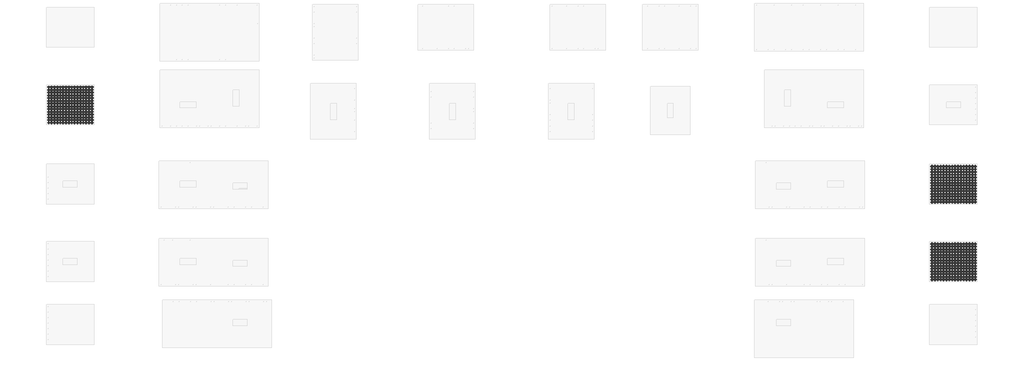
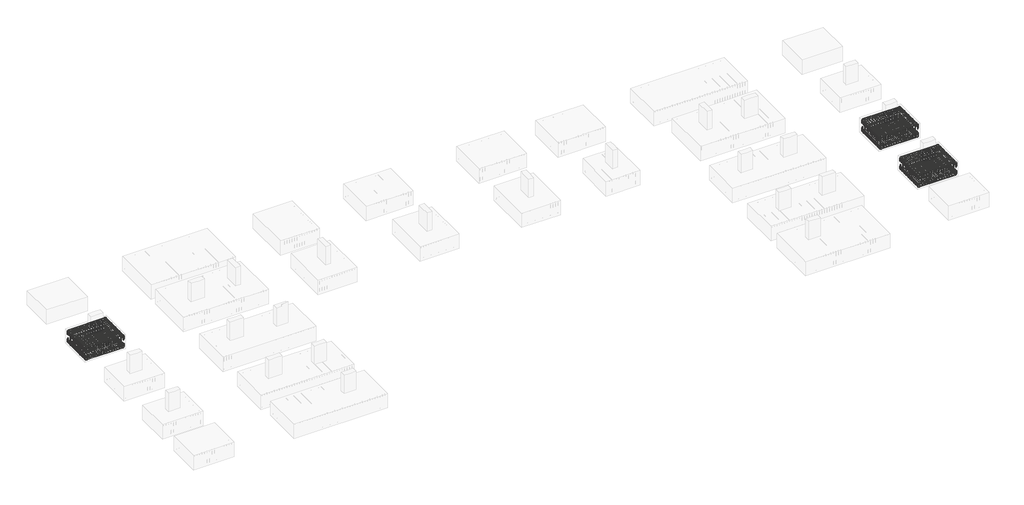
# One storey, part 9 of 21: 12 reinforcing bars.
"""IFC4 building model written with IfcOpenShell, lengths in millimetres."""

from ifc_helpers import new_model, si_unit, point, frame, origin, place, context, project, spatial, polyline, circle_curve, trimmed, segment, composite_curve, source, transform, mapped, element, save
from ifc_brep_helpers import swept_disk

model = new_model("IFC4")

# Units and contexts
model_context = context("Model", 3, world=origin())
ifc_project = project(units=[si_unit("LENGTHUNIT", "METRE", prefix="MILLI")], contexts=[model_context])

# Site, building, storey
site = spatial("IfcSite", under=ifc_project)
building = spatial("IfcBuilding", under=site)
storey = spatial("IfcBuildingStorey", under=building, Elevation=-1100.0)

# Reinforcing bars
placement = place(None, origin())
reinforcing_bar_shape = source(origin(), model_context, "Body", "SolidModel", [
    swept_disk(composite_curve([segment(polyline([(-23061.1351198, 4447.9216575, -1700.0), (-23061.1351198, 4447.9216575, -1882.5)]), True, "CONTINUOUS"), segment(trimmed(circle_curve(frame((-23118.6351198, 4447.9216575, -1882.5), z_axis=(0.0, 1.0, 0.0), x_axis=(57.5, 0.0, 0.0)), 57.5), [point((-23061.1351198, 4447.9216575, -1882.5))], [point((-23118.6351198, 4447.9216575, -1940.0))], True, "CARTESIAN"), True, "CONTINUOUS"), segment(polyline([(-23118.6351198, 4447.9216575, -1940.0), (-25283.6351198, 4447.9216575, -1940.0)]), True, "CONTINUOUS"), segment(trimmed(circle_curve(frame((-25283.6351198, 4447.9216575, -1882.5), z_axis=(0.0, 1.0, 0.0), x_axis=(0.0, 0.0, -57.5)), 57.5), [point((-25283.6351198, 4447.9216575, -1940.0))], [point((-25341.1351198, 4447.9216575, -1882.5))], True, "CARTESIAN"), True, "CONTINUOUS"), segment(polyline([(-25341.1351198, 4447.9216575, -1882.5), (-25341.1351198, 4447.9216575, -1700.0)]), True, "CONTINUOUS")], self_intersect=False), 10.0),
])
element("IfcReinforcingBar", 1, at=placement, inside=storey, context=model_context, shape_type="MappedRepresentation", body=[
    mapped(reinforcing_bar_shape, transform((0.0, 0.0, 0.0), x_axis=(1.0, 0.0, 0.0), y_axis=(0.0, 1.0, 0.0), z_axis=(0.0, 0.0, 1.0))),
    mapped(reinforcing_bar_shape, transform((0.0, -138.5928916, 0.0), x_axis=(1.0, 0.0, 0.0), y_axis=(0.0, 1.0, 0.0), z_axis=(0.0, 0.0, 1.0))),
    mapped(reinforcing_bar_shape, transform((0.0, -277.1857833, 0.0), x_axis=(1.0, 0.0, 0.0), y_axis=(0.0, 1.0, 0.0), z_axis=(0.0, 0.0, 1.0))),
    mapped(reinforcing_bar_shape, transform((0.0, -415.7786749, 0.0), x_axis=(1.0, 0.0, 0.0), y_axis=(0.0, 1.0, 0.0), z_axis=(0.0, 0.0, 1.0))),
    mapped(reinforcing_bar_shape, transform((0.0, -554.3715666, 0.0), x_axis=(1.0, 0.0, 0.0), y_axis=(0.0, 1.0, 0.0), z_axis=(0.0, 0.0, 1.0))),
    mapped(reinforcing_bar_shape, transform((0.0, -692.9644582, 0.0), x_axis=(1.0, 0.0, 0.0), y_axis=(0.0, 1.0, 0.0), z_axis=(0.0, 0.0, 1.0))),
    mapped(reinforcing_bar_shape, transform((0.0, -831.5573499, 0.0), x_axis=(1.0, 0.0, 0.0), y_axis=(0.0, 1.0, 0.0), z_axis=(0.0, 0.0, 1.0))),
    mapped(reinforcing_bar_shape, transform((0.0, -970.1502415, 0.0), x_axis=(1.0, 0.0, 0.0), y_axis=(0.0, 1.0, 0.0), z_axis=(0.0, 0.0, 1.0))),
    mapped(reinforcing_bar_shape, transform((0.0, -1108.7431331, 0.0), x_axis=(1.0, 0.0, 0.0), y_axis=(0.0, 1.0, 0.0), z_axis=(0.0, 0.0, 1.0))),
    mapped(reinforcing_bar_shape, transform((0.0, -1247.3360248, 0.0), x_axis=(1.0, 0.0, 0.0), y_axis=(0.0, 1.0, 0.0), z_axis=(0.0, 0.0, 1.0))),
    mapped(reinforcing_bar_shape, transform((0.0, -1385.9289164, 0.0), x_axis=(1.0, 0.0, 0.0), y_axis=(0.0, 1.0, 0.0), z_axis=(0.0, 0.0, 1.0))),
    mapped(reinforcing_bar_shape, transform((0.0, -1524.5218081, 0.0), x_axis=(1.0, 0.0, 0.0), y_axis=(0.0, 1.0, 0.0), z_axis=(0.0, 0.0, 1.0))),
    mapped(reinforcing_bar_shape, transform((0.0, -1663.1146997, 0.0), x_axis=(1.0, 0.0, 0.0), y_axis=(0.0, 1.0, 0.0), z_axis=(0.0, 0.0, 1.0))),
    mapped(reinforcing_bar_shape, transform((0.0, -1801.7075913, 0.0), x_axis=(1.0, 0.0, 0.0), y_axis=(0.0, 1.0, 0.0), z_axis=(0.0, 0.0, 1.0))),
])
reinforcing_bar_2_shape = source(origin(), model_context, "Body", "SolidModel", [
    swept_disk(composite_curve([segment(polyline([(-25343.1851198, 4447.9216575, -1400.0), (-25343.1851198, 4447.9216575, -1213.4)]), True, "CONTINUOUS"), segment(trimmed(circle_curve(frame((-25287.7351198, 4447.9216575, -1213.4), z_axis=(0.0, 1.0, 0.0), x_axis=(-55.45000000000073, 0.0, 0.0)), 55.45), [point((-25343.1851198, 4447.9216575, -1213.4))], [point((-25287.7351198, 4447.9216575, -1157.95))], True, "CARTESIAN"), True, "CONTINUOUS"), segment(polyline([(-25287.7351198, 4447.9216575, -1157.95), (-23114.5351198, 4447.9216575, -1157.95)]), True, "CONTINUOUS"), segment(trimmed(circle_curve(frame((-23114.5351198, 4447.9216575, -1213.4), z_axis=(0.0, 1.0, 0.0), x_axis=(0.0, 0.0, 55.450000000000045)), 55.45), [point((-23114.5351198, 4447.9216575, -1157.95))], [point((-23059.0851198, 4447.9216575, -1213.4))], True, "CARTESIAN"), True, "CONTINUOUS"), segment(polyline([(-23059.0851198, 4447.9216575, -1213.4), (-23059.0851198, 4447.9216575, -1400.0)]), True, "CONTINUOUS")], self_intersect=False), 7.95),
])
element("IfcReinforcingBar", 2, at=placement, inside=storey, context=model_context, shape_type="MappedRepresentation", body=[
    mapped(reinforcing_bar_2_shape, transform((0.0, 0.0, 0.0), x_axis=(1.0, 0.0, 0.0), y_axis=(0.0, 1.0, 0.0), z_axis=(0.0, 0.0, 1.0))),
    mapped(reinforcing_bar_2_shape, transform((0.0, -138.5928916, 0.0), x_axis=(1.0, 0.0, 0.0), y_axis=(0.0, 1.0, 0.0), z_axis=(0.0, 0.0, 1.0))),
    mapped(reinforcing_bar_2_shape, transform((0.0, -277.1857833, 0.0), x_axis=(1.0, 0.0, 0.0), y_axis=(0.0, 1.0, 0.0), z_axis=(0.0, 0.0, 1.0))),
    mapped(reinforcing_bar_2_shape, transform((0.0, -415.7786749, 0.0), x_axis=(1.0, 0.0, 0.0), y_axis=(0.0, 1.0, 0.0), z_axis=(0.0, 0.0, 1.0))),
    mapped(reinforcing_bar_2_shape, transform((0.0, -554.3715666, 0.0), x_axis=(1.0, 0.0, 0.0), y_axis=(0.0, 1.0, 0.0), z_axis=(0.0, 0.0, 1.0))),
    mapped(reinforcing_bar_2_shape, transform((0.0, -692.9644582, 0.0), x_axis=(1.0, 0.0, 0.0), y_axis=(0.0, 1.0, 0.0), z_axis=(0.0, 0.0, 1.0))),
    mapped(reinforcing_bar_2_shape, transform((0.0, -831.5573499, 0.0), x_axis=(1.0, 0.0, 0.0), y_axis=(0.0, 1.0, 0.0), z_axis=(0.0, 0.0, 1.0))),
    mapped(reinforcing_bar_2_shape, transform((0.0, -970.1502415, 0.0), x_axis=(1.0, 0.0, 0.0), y_axis=(0.0, 1.0, 0.0), z_axis=(0.0, 0.0, 1.0))),
    mapped(reinforcing_bar_2_shape, transform((0.0, -1108.7431331, 0.0), x_axis=(1.0, 0.0, 0.0), y_axis=(0.0, 1.0, 0.0), z_axis=(0.0, 0.0, 1.0))),
    mapped(reinforcing_bar_2_shape, transform((0.0, -1247.3360248, 0.0), x_axis=(1.0, 0.0, 0.0), y_axis=(0.0, 1.0, 0.0), z_axis=(0.0, 0.0, 1.0))),
    mapped(reinforcing_bar_2_shape, transform((0.0, -1385.9289164, 0.0), x_axis=(1.0, 0.0, 0.0), y_axis=(0.0, 1.0, 0.0), z_axis=(0.0, 0.0, 1.0))),
    mapped(reinforcing_bar_2_shape, transform((0.0, -1524.5218081, 0.0), x_axis=(1.0, 0.0, 0.0), y_axis=(0.0, 1.0, 0.0), z_axis=(0.0, 0.0, 1.0))),
    mapped(reinforcing_bar_2_shape, transform((0.0, -1663.1146997, 0.0), x_axis=(1.0, 0.0, 0.0), y_axis=(0.0, 1.0, 0.0), z_axis=(0.0, 0.0, 1.0))),
    mapped(reinforcing_bar_2_shape, transform((0.0, -1801.7075913, 0.0), x_axis=(1.0, 0.0, 0.0), y_axis=(0.0, 1.0, 0.0), z_axis=(0.0, 0.0, 1.0))),
])
reinforcing_bar_3_shape = source(origin(), model_context, "Body", "SolidModel", [
    swept_disk(composite_curve([segment(polyline([(-23110.9192838, 4486.2204288, -1428.1111113), (-23110.9192838, 4486.2204288, -1241.5111113)]), True, "CONTINUOUS"), segment(trimmed(circle_curve(frame((-23110.9192838, 4430.7704288, -1241.5111113), z_axis=(1.0, 0.0, 0.0), x_axis=(0.0, 55.44999999999982, 0.0)), 55.45), [point((-23110.9192838, 4486.2204288, -1241.5111113))], [point((-23110.9192838, 4430.7704288, -1186.0611113))], True, "CARTESIAN"), True, "CONTINUOUS"), segment(polyline([(-23110.9192838, 4430.7704288, -1186.0611113), (-23110.9192838, 2657.5704288, -1186.0611113)]), True, "CONTINUOUS"), segment(trimmed(circle_curve(frame((-23110.9192838, 2657.5704288, -1241.5111113), z_axis=(1.0, 0.0, 0.0), x_axis=(0.0, 0.0, 55.450000000000045)), 55.45), [point((-23110.9192838, 2657.5704288, -1186.0611113))], [point((-23110.9192838, 2602.1204288, -1241.5111113))], True, "CARTESIAN"), True, "CONTINUOUS"), segment(polyline([(-23110.9192838, 2602.1204288, -1241.5111113), (-23110.9192838, 2602.1204288, -1428.1111113)]), True, "CONTINUOUS")], self_intersect=False), 7.95),
])
element("IfcReinforcingBar", 3, at=placement, inside=storey, context=model_context, shape_type="MappedRepresentation", body=[
    mapped(reinforcing_bar_3_shape, transform((0.0, 0.0, 0.0), x_axis=(1.0, 0.0, 0.0), y_axis=(0.0, 1.0, 0.0), z_axis=(0.0, 0.0, 1.0))),
    mapped(reinforcing_bar_3_shape, transform((-145.2528929, 0.0, 0.0), x_axis=(1.0, 0.0, 0.0), y_axis=(0.0, 1.0, 0.0), z_axis=(0.0, 0.0, 1.0))),
    mapped(reinforcing_bar_3_shape, transform((-290.5057858, 0.0, 0.0), x_axis=(1.0, 0.0, 0.0), y_axis=(0.0, 1.0, 0.0), z_axis=(0.0, 0.0, 1.0))),
    mapped(reinforcing_bar_3_shape, transform((-435.7586787, 0.0, 0.0), x_axis=(1.0, 0.0, 0.0), y_axis=(0.0, 1.0, 0.0), z_axis=(0.0, 0.0, 1.0))),
    mapped(reinforcing_bar_3_shape, transform((-581.0115716, 0.0, 0.0), x_axis=(1.0, 0.0, 0.0), y_axis=(0.0, 1.0, 0.0), z_axis=(0.0, 0.0, 1.0))),
    mapped(reinforcing_bar_3_shape, transform((-726.2644645, 0.0, 0.0), x_axis=(1.0, 0.0, 0.0), y_axis=(0.0, 1.0, 0.0), z_axis=(0.0, 0.0, 1.0))),
    mapped(reinforcing_bar_3_shape, transform((-871.5173574, 0.0, 0.0), x_axis=(1.0, 0.0, 0.0), y_axis=(0.0, 1.0, 0.0), z_axis=(0.0, 0.0, 1.0))),
    mapped(reinforcing_bar_3_shape, transform((-1016.7702503, 0.0, 0.0), x_axis=(1.0, 0.0, 0.0), y_axis=(0.0, 1.0, 0.0), z_axis=(0.0, 0.0, 1.0))),
    mapped(reinforcing_bar_3_shape, transform((-1162.0231432, 0.0, 0.0), x_axis=(1.0, 0.0, 0.0), y_axis=(0.0, 1.0, 0.0), z_axis=(0.0, 0.0, 1.0))),
    mapped(reinforcing_bar_3_shape, transform((-1307.276036, 0.0, 0.0), x_axis=(1.0, 0.0, 0.0), y_axis=(0.0, 1.0, 0.0), z_axis=(0.0, 0.0, 1.0))),
    mapped(reinforcing_bar_3_shape, transform((-1452.5289289, 0.0, 0.0), x_axis=(1.0, 0.0, 0.0), y_axis=(0.0, 1.0, 0.0), z_axis=(0.0, 0.0, 1.0))),
    mapped(reinforcing_bar_3_shape, transform((-1597.7818218, 0.0, 0.0), x_axis=(1.0, 0.0, 0.0), y_axis=(0.0, 1.0, 0.0), z_axis=(0.0, 0.0, 1.0))),
    mapped(reinforcing_bar_3_shape, transform((-1743.0347147, 0.0, 0.0), x_axis=(1.0, 0.0, 0.0), y_axis=(0.0, 1.0, 0.0), z_axis=(0.0, 0.0, 1.0))),
    mapped(reinforcing_bar_3_shape, transform((-1888.2876076, 0.0, 0.0), x_axis=(1.0, 0.0, 0.0), y_axis=(0.0, 1.0, 0.0), z_axis=(0.0, 0.0, 1.0))),
    mapped(reinforcing_bar_3_shape, transform((-2033.5405005, 0.0, 0.0), x_axis=(1.0, 0.0, 0.0), y_axis=(0.0, 1.0, 0.0), z_axis=(0.0, 0.0, 1.0))),
    mapped(reinforcing_bar_3_shape, transform((-2178.7933934, 0.0, 0.0), x_axis=(1.0, 0.0, 0.0), y_axis=(0.0, 1.0, 0.0), z_axis=(0.0, 0.0, 1.0))),
])
reinforcing_bar_4_shape = source(origin(), model_context, "Body", "SolidModel", [
    swept_disk(composite_curve([segment(polyline([(-25289.7126773, 4484.1704288, -1669.8442859), (-25289.7126773, 4484.1704288, -1852.3442859)]), True, "CONTINUOUS"), segment(trimmed(circle_curve(frame((-25289.7126773, 4426.6704288, -1852.3442859), z_axis=(-1.0, 0.0, 0.0), x_axis=(0.0, 57.5, 0.0)), 57.5), [point((-25289.7126773, 4484.1704288, -1852.3442859))], [point((-25289.7126773, 4426.6704288, -1909.8442859))], True, "CARTESIAN"), True, "CONTINUOUS"), segment(polyline([(-25289.7126773, 4426.6704288, -1909.8442859), (-25289.7126773, 2661.6704288, -1909.8442859)]), True, "CONTINUOUS"), segment(trimmed(circle_curve(frame((-25289.7126773, 2661.6704288, -1852.3442859), z_axis=(-1.0, 0.0, 0.0), x_axis=(0.0, 0.0, -57.5)), 57.5), [point((-25289.7126773, 2661.6704288, -1909.8442859))], [point((-25289.7126773, 2604.1704288, -1852.3442859))], True, "CARTESIAN"), True, "CONTINUOUS"), segment(polyline([(-25289.7126773, 2604.1704288, -1852.3442859), (-25289.7126773, 2604.1704288, -1669.8442859)]), True, "CONTINUOUS")], self_intersect=False), 10.0),
])
element("IfcReinforcingBar", 4, at=placement, inside=storey, context=model_context, shape_type="MappedRepresentation", body=[
    mapped(reinforcing_bar_4_shape, transform((0.0, 0.0, 0.0), x_axis=(1.0, 0.0, 0.0), y_axis=(0.0, 1.0, 0.0), z_axis=(0.0, 0.0, 1.0))),
    mapped(reinforcing_bar_4_shape, transform((145.2528929, 0.0, 0.0), x_axis=(1.0, 0.0, 0.0), y_axis=(0.0, 1.0, 0.0), z_axis=(0.0, 0.0, 1.0))),
    mapped(reinforcing_bar_4_shape, transform((290.5057858, 0.0, 0.0), x_axis=(1.0, 0.0, 0.0), y_axis=(0.0, 1.0, 0.0), z_axis=(0.0, 0.0, 1.0))),
    mapped(reinforcing_bar_4_shape, transform((435.7586787, 0.0, 0.0), x_axis=(1.0, 0.0, 0.0), y_axis=(0.0, 1.0, 0.0), z_axis=(0.0, 0.0, 1.0))),
    mapped(reinforcing_bar_4_shape, transform((581.0115716, 0.0, 0.0), x_axis=(1.0, 0.0, 0.0), y_axis=(0.0, 1.0, 0.0), z_axis=(0.0, 0.0, 1.0))),
    mapped(reinforcing_bar_4_shape, transform((726.2644645, 0.0, 0.0), x_axis=(1.0, 0.0, 0.0), y_axis=(0.0, 1.0, 0.0), z_axis=(0.0, 0.0, 1.0))),
    mapped(reinforcing_bar_4_shape, transform((871.5173574, 0.0, 0.0), x_axis=(1.0, 0.0, 0.0), y_axis=(0.0, 1.0, 0.0), z_axis=(0.0, 0.0, 1.0))),
    mapped(reinforcing_bar_4_shape, transform((1016.7702503, 0.0, 0.0), x_axis=(1.0, 0.0, 0.0), y_axis=(0.0, 1.0, 0.0), z_axis=(0.0, 0.0, 1.0))),
    mapped(reinforcing_bar_4_shape, transform((1162.0231432, 0.0, 0.0), x_axis=(1.0, 0.0, 0.0), y_axis=(0.0, 1.0, 0.0), z_axis=(0.0, 0.0, 1.0))),
    mapped(reinforcing_bar_4_shape, transform((1307.276036, 0.0, 0.0), x_axis=(1.0, 0.0, 0.0), y_axis=(0.0, 1.0, 0.0), z_axis=(0.0, 0.0, 1.0))),
    mapped(reinforcing_bar_4_shape, transform((1452.5289289, 0.0, 0.0), x_axis=(1.0, 0.0, 0.0), y_axis=(0.0, 1.0, 0.0), z_axis=(0.0, 0.0, 1.0))),
    mapped(reinforcing_bar_4_shape, transform((1597.7818218, 0.0, 0.0), x_axis=(1.0, 0.0, 0.0), y_axis=(0.0, 1.0, 0.0), z_axis=(0.0, 0.0, 1.0))),
    mapped(reinforcing_bar_4_shape, transform((1743.0347147, 0.0, 0.0), x_axis=(1.0, 0.0, 0.0), y_axis=(0.0, 1.0, 0.0), z_axis=(0.0, 0.0, 1.0))),
    mapped(reinforcing_bar_4_shape, transform((1888.2876076, 0.0, 0.0), x_axis=(1.0, 0.0, 0.0), y_axis=(0.0, 1.0, 0.0), z_axis=(0.0, 0.0, 1.0))),
    mapped(reinforcing_bar_4_shape, transform((2033.5405005, 0.0, 0.0), x_axis=(1.0, 0.0, 0.0), y_axis=(0.0, 1.0, 0.0), z_axis=(0.0, 0.0, 1.0))),
    mapped(reinforcing_bar_4_shape, transform((2178.7933934, 0.0, 0.0), x_axis=(1.0, 0.0, 0.0), y_axis=(0.0, 1.0, 0.0), z_axis=(0.0, 0.0, 1.0))),
])
reinforcing_bar_5_shape = source(origin(), model_context, "Body", "SolidModel", [
    swept_disk(composite_curve([segment(polyline([(19239.1673659, -5269.5807999, -1700.0), (19239.1673659, -5269.5807999, -1882.5)]), True, "CONTINUOUS"), segment(trimmed(circle_curve(frame((19296.6673659, -5269.5807999, -1882.5), z_axis=(0.0, -1.0, 0.0), x_axis=(-57.5, 0.0, 0.0)), 57.5), [point((19239.1673659, -5269.5807999, -1882.5))], [point((19296.6673659, -5269.5807999, -1940.0))], True, "CARTESIAN"), True, "CONTINUOUS"), segment(polyline([(19296.6673659, -5269.5807999, -1940.0), (21461.6673659, -5269.5807999, -1940.0)]), True, "CONTINUOUS"), segment(trimmed(circle_curve(frame((21461.6673659, -5269.5807999, -1882.5), z_axis=(0.0, -1.0, 0.0), x_axis=(0.0, 0.0, -57.5)), 57.5), [point((21461.6673659, -5269.5807999, -1940.0))], [point((21519.1673659, -5269.5807999, -1882.5))], True, "CARTESIAN"), True, "CONTINUOUS"), segment(polyline([(21519.1673659, -5269.5807999, -1882.5), (21519.1673659, -5269.5807999, -1700.0)]), True, "CONTINUOUS")], self_intersect=False), 10.0),
])
element("IfcReinforcingBar", 5, at=placement, inside=storey, context=model_context, shape_type="MappedRepresentation", body=[
    mapped(reinforcing_bar_5_shape, transform((0.0, 0.0, 0.0), x_axis=(1.0, 0.0, 0.0), y_axis=(0.0, 1.0, 0.0), z_axis=(0.0, 0.0, 1.0))),
    mapped(reinforcing_bar_5_shape, transform((0.0, 138.5928916, 0.0), x_axis=(1.0, 0.0, 0.0), y_axis=(0.0, 1.0, 0.0), z_axis=(0.0, 0.0, 1.0))),
    mapped(reinforcing_bar_5_shape, transform((0.0, 277.1857833, 0.0), x_axis=(1.0, 0.0, 0.0), y_axis=(0.0, 1.0, 0.0), z_axis=(0.0, 0.0, 1.0))),
    mapped(reinforcing_bar_5_shape, transform((0.0, 415.7786749, 0.0), x_axis=(1.0, 0.0, 0.0), y_axis=(0.0, 1.0, 0.0), z_axis=(0.0, 0.0, 1.0))),
    mapped(reinforcing_bar_5_shape, transform((0.0, 554.3715666, 0.0), x_axis=(1.0, 0.0, 0.0), y_axis=(0.0, 1.0, 0.0), z_axis=(0.0, 0.0, 1.0))),
    mapped(reinforcing_bar_5_shape, transform((0.0, 692.9644582, 0.0), x_axis=(1.0, 0.0, 0.0), y_axis=(0.0, 1.0, 0.0), z_axis=(0.0, 0.0, 1.0))),
    mapped(reinforcing_bar_5_shape, transform((0.0, 831.5573499, 0.0), x_axis=(1.0, 0.0, 0.0), y_axis=(0.0, 1.0, 0.0), z_axis=(0.0, 0.0, 1.0))),
    mapped(reinforcing_bar_5_shape, transform((0.0, 970.1502415, 0.0), x_axis=(1.0, 0.0, 0.0), y_axis=(0.0, 1.0, 0.0), z_axis=(0.0, 0.0, 1.0))),
    mapped(reinforcing_bar_5_shape, transform((0.0, 1108.7431331, 0.0), x_axis=(1.0, 0.0, 0.0), y_axis=(0.0, 1.0, 0.0), z_axis=(0.0, 0.0, 1.0))),
    mapped(reinforcing_bar_5_shape, transform((0.0, 1247.3360248, 0.0), x_axis=(1.0, 0.0, 0.0), y_axis=(0.0, 1.0, 0.0), z_axis=(0.0, 0.0, 1.0))),
    mapped(reinforcing_bar_5_shape, transform((0.0, 1385.9289164, 0.0), x_axis=(1.0, 0.0, 0.0), y_axis=(0.0, 1.0, 0.0), z_axis=(0.0, 0.0, 1.0))),
    mapped(reinforcing_bar_5_shape, transform((0.0, 1524.5218081, 0.0), x_axis=(1.0, 0.0, 0.0), y_axis=(0.0, 1.0, 0.0), z_axis=(0.0, 0.0, 1.0))),
    mapped(reinforcing_bar_5_shape, transform((0.0, 1663.1146997, 0.0), x_axis=(1.0, 0.0, 0.0), y_axis=(0.0, 1.0, 0.0), z_axis=(0.0, 0.0, 1.0))),
    mapped(reinforcing_bar_5_shape, transform((0.0, 1801.7075913, 0.0), x_axis=(1.0, 0.0, 0.0), y_axis=(0.0, 1.0, 0.0), z_axis=(0.0, 0.0, 1.0))),
])
reinforcing_bar_6_shape = source(origin(), model_context, "Body", "SolidModel", [
    swept_disk(composite_curve([segment(polyline([(21521.2173659, -5269.5807999, -1400.0), (21521.2173659, -5269.5807999, -1213.4)]), True, "CONTINUOUS"), segment(trimmed(circle_curve(frame((21465.7673659, -5269.5807999, -1213.4), z_axis=(0.0, -1.0, 0.0), x_axis=(55.45000000000073, 0.0, 0.0)), 55.45), [point((21521.2173659, -5269.5807999, -1213.4))], [point((21465.7673659, -5269.5807999, -1157.95))], True, "CARTESIAN"), True, "CONTINUOUS"), segment(polyline([(21465.7673659, -5269.5807999, -1157.95), (19292.5673659, -5269.5807999, -1157.95)]), True, "CONTINUOUS"), segment(trimmed(circle_curve(frame((19292.5673659, -5269.5807999, -1213.4), z_axis=(0.0, -1.0, 0.0), x_axis=(0.0, 0.0, 55.450000000000045)), 55.45), [point((19292.5673659, -5269.5807999, -1157.95))], [point((19237.1173659, -5269.5807999, -1213.4))], True, "CARTESIAN"), True, "CONTINUOUS"), segment(polyline([(19237.1173659, -5269.5807999, -1213.4), (19237.1173659, -5269.5807999, -1400.0)]), True, "CONTINUOUS")], self_intersect=False), 7.95),
])
element("IfcReinforcingBar", 6, at=placement, inside=storey, context=model_context, shape_type="MappedRepresentation", body=[
    mapped(reinforcing_bar_6_shape, transform((0.0, 0.0, 0.0), x_axis=(1.0, 0.0, 0.0), y_axis=(0.0, 1.0, 0.0), z_axis=(0.0, 0.0, 1.0))),
    mapped(reinforcing_bar_6_shape, transform((0.0, 138.5928916, 0.0), x_axis=(1.0, 0.0, 0.0), y_axis=(0.0, 1.0, 0.0), z_axis=(0.0, 0.0, 1.0))),
    mapped(reinforcing_bar_6_shape, transform((0.0, 277.1857833, 0.0), x_axis=(1.0, 0.0, 0.0), y_axis=(0.0, 1.0, 0.0), z_axis=(0.0, 0.0, 1.0))),
    mapped(reinforcing_bar_6_shape, transform((0.0, 415.7786749, 0.0), x_axis=(1.0, 0.0, 0.0), y_axis=(0.0, 1.0, 0.0), z_axis=(0.0, 0.0, 1.0))),
    mapped(reinforcing_bar_6_shape, transform((0.0, 554.3715666, 0.0), x_axis=(1.0, 0.0, 0.0), y_axis=(0.0, 1.0, 0.0), z_axis=(0.0, 0.0, 1.0))),
    mapped(reinforcing_bar_6_shape, transform((0.0, 692.9644582, 0.0), x_axis=(1.0, 0.0, 0.0), y_axis=(0.0, 1.0, 0.0), z_axis=(0.0, 0.0, 1.0))),
    mapped(reinforcing_bar_6_shape, transform((0.0, 831.5573499, 0.0), x_axis=(1.0, 0.0, 0.0), y_axis=(0.0, 1.0, 0.0), z_axis=(0.0, 0.0, 1.0))),
    mapped(reinforcing_bar_6_shape, transform((0.0, 970.1502415, 0.0), x_axis=(1.0, 0.0, 0.0), y_axis=(0.0, 1.0, 0.0), z_axis=(0.0, 0.0, 1.0))),
    mapped(reinforcing_bar_6_shape, transform((0.0, 1108.7431331, 0.0), x_axis=(1.0, 0.0, 0.0), y_axis=(0.0, 1.0, 0.0), z_axis=(0.0, 0.0, 1.0))),
    mapped(reinforcing_bar_6_shape, transform((0.0, 1247.3360248, 0.0), x_axis=(1.0, 0.0, 0.0), y_axis=(0.0, 1.0, 0.0), z_axis=(0.0, 0.0, 1.0))),
    mapped(reinforcing_bar_6_shape, transform((0.0, 1385.9289164, 0.0), x_axis=(1.0, 0.0, 0.0), y_axis=(0.0, 1.0, 0.0), z_axis=(0.0, 0.0, 1.0))),
    mapped(reinforcing_bar_6_shape, transform((0.0, 1524.5218081, 0.0), x_axis=(1.0, 0.0, 0.0), y_axis=(0.0, 1.0, 0.0), z_axis=(0.0, 0.0, 1.0))),
    mapped(reinforcing_bar_6_shape, transform((0.0, 1663.1146997, 0.0), x_axis=(1.0, 0.0, 0.0), y_axis=(0.0, 1.0, 0.0), z_axis=(0.0, 0.0, 1.0))),
    mapped(reinforcing_bar_6_shape, transform((0.0, 1801.7075913, 0.0), x_axis=(1.0, 0.0, 0.0), y_axis=(0.0, 1.0, 0.0), z_axis=(0.0, 0.0, 1.0))),
])
reinforcing_bar_7_shape = source(origin(), model_context, "Body", "SolidModel", [
    swept_disk(composite_curve([segment(polyline([(19288.9515299, -5307.8795712, -1428.1111113), (19288.9515299, -5307.8795712, -1241.5111113)]), True, "CONTINUOUS"), segment(trimmed(circle_curve(frame((19288.9515299, -5252.4295712, -1241.5111113), z_axis=(-1.0, 0.0, 0.0), x_axis=(0.0, -55.44999999999982, 0.0)), 55.45), [point((19288.9515299, -5307.8795712, -1241.5111113))], [point((19288.9515299, -5252.4295712, -1186.0611113))], True, "CARTESIAN"), True, "CONTINUOUS"), segment(polyline([(19288.9515299, -5252.4295712, -1186.0611113), (19288.9515299, -3479.2295712, -1186.0611113)]), True, "CONTINUOUS"), segment(trimmed(circle_curve(frame((19288.9515299, -3479.2295712, -1241.5111113), z_axis=(-1.0, 0.0, 0.0), x_axis=(0.0, 0.0, 55.450000000000045)), 55.45), [point((19288.9515299, -3479.2295712, -1186.0611113))], [point((19288.9515299, -3423.7795712, -1241.5111113))], True, "CARTESIAN"), True, "CONTINUOUS"), segment(polyline([(19288.9515299, -3423.7795712, -1241.5111113), (19288.9515299, -3423.7795712, -1428.1111113)]), True, "CONTINUOUS")], self_intersect=False), 7.95),
])
element("IfcReinforcingBar", 7, at=placement, inside=storey, context=model_context, shape_type="MappedRepresentation", body=[
    mapped(reinforcing_bar_7_shape, transform((0.0, 0.0, 0.0), x_axis=(1.0, 0.0, 0.0), y_axis=(0.0, 1.0, 0.0), z_axis=(0.0, 0.0, 1.0))),
    mapped(reinforcing_bar_7_shape, transform((145.2528929, 0.0, 0.0), x_axis=(1.0, 0.0, 0.0), y_axis=(0.0, 1.0, 0.0), z_axis=(0.0, 0.0, 1.0))),
    mapped(reinforcing_bar_7_shape, transform((290.5057858, 0.0, 0.0), x_axis=(1.0, 0.0, 0.0), y_axis=(0.0, 1.0, 0.0), z_axis=(0.0, 0.0, 1.0))),
    mapped(reinforcing_bar_7_shape, transform((435.7586787, 0.0, 0.0), x_axis=(1.0, 0.0, 0.0), y_axis=(0.0, 1.0, 0.0), z_axis=(0.0, 0.0, 1.0))),
    mapped(reinforcing_bar_7_shape, transform((581.0115716, 0.0, 0.0), x_axis=(1.0, 0.0, 0.0), y_axis=(0.0, 1.0, 0.0), z_axis=(0.0, 0.0, 1.0))),
    mapped(reinforcing_bar_7_shape, transform((726.2644645, 0.0, 0.0), x_axis=(1.0, 0.0, 0.0), y_axis=(0.0, 1.0, 0.0), z_axis=(0.0, 0.0, 1.0))),
    mapped(reinforcing_bar_7_shape, transform((871.5173574, 0.0, 0.0), x_axis=(1.0, 0.0, 0.0), y_axis=(0.0, 1.0, 0.0), z_axis=(0.0, 0.0, 1.0))),
    mapped(reinforcing_bar_7_shape, transform((1016.7702503, 0.0, 0.0), x_axis=(1.0, 0.0, 0.0), y_axis=(0.0, 1.0, 0.0), z_axis=(0.0, 0.0, 1.0))),
    mapped(reinforcing_bar_7_shape, transform((1162.0231432, 0.0, 0.0), x_axis=(1.0, 0.0, 0.0), y_axis=(0.0, 1.0, 0.0), z_axis=(0.0, 0.0, 1.0))),
    mapped(reinforcing_bar_7_shape, transform((1307.276036, 0.0, 0.0), x_axis=(1.0, 0.0, 0.0), y_axis=(0.0, 1.0, 0.0), z_axis=(0.0, 0.0, 1.0))),
    mapped(reinforcing_bar_7_shape, transform((1452.5289289, 0.0, 0.0), x_axis=(1.0, 0.0, 0.0), y_axis=(0.0, 1.0, 0.0), z_axis=(0.0, 0.0, 1.0))),
    mapped(reinforcing_bar_7_shape, transform((1597.7818218, 0.0, 0.0), x_axis=(1.0, 0.0, 0.0), y_axis=(0.0, 1.0, 0.0), z_axis=(0.0, 0.0, 1.0))),
    mapped(reinforcing_bar_7_shape, transform((1743.0347147, 0.0, 0.0), x_axis=(1.0, 0.0, 0.0), y_axis=(0.0, 1.0, 0.0), z_axis=(0.0, 0.0, 1.0))),
    mapped(reinforcing_bar_7_shape, transform((1888.2876076, 0.0, 0.0), x_axis=(1.0, 0.0, 0.0), y_axis=(0.0, 1.0, 0.0), z_axis=(0.0, 0.0, 1.0))),
    mapped(reinforcing_bar_7_shape, transform((2033.5405005, 0.0, 0.0), x_axis=(1.0, 0.0, 0.0), y_axis=(0.0, 1.0, 0.0), z_axis=(0.0, 0.0, 1.0))),
    mapped(reinforcing_bar_7_shape, transform((2178.7933934, 0.0, 0.0), x_axis=(1.0, 0.0, 0.0), y_axis=(0.0, 1.0, 0.0), z_axis=(0.0, 0.0, 1.0))),
])
reinforcing_bar_8_shape = source(origin(), model_context, "Body", "SolidModel", [
    swept_disk(composite_curve([segment(polyline([(21467.7449233, -5305.8295712, -1669.8442859), (21467.7449233, -5305.8295712, -1852.3442859)]), True, "CONTINUOUS"), segment(trimmed(circle_curve(frame((21467.7449233, -5248.3295712, -1852.3442859), z_axis=(1.0, 0.0, 0.0), x_axis=(0.0, -57.5, 0.0)), 57.5), [point((21467.7449233, -5305.8295712, -1852.3442859))], [point((21467.7449233, -5248.3295712, -1909.8442859))], True, "CARTESIAN"), True, "CONTINUOUS"), segment(polyline([(21467.7449233, -5248.3295712, -1909.8442859), (21467.7449233, -3483.3295712, -1909.8442859)]), True, "CONTINUOUS"), segment(trimmed(circle_curve(frame((21467.7449233, -3483.3295712, -1852.3442859), z_axis=(1.0, 0.0, 0.0), x_axis=(0.0, 0.0, -57.5)), 57.5), [point((21467.7449233, -3483.3295712, -1909.8442859))], [point((21467.7449233, -3425.8295712, -1852.3442859))], True, "CARTESIAN"), True, "CONTINUOUS"), segment(polyline([(21467.7449233, -3425.8295712, -1852.3442859), (21467.7449233, -3425.8295712, -1669.8442859)]), True, "CONTINUOUS")], self_intersect=False), 10.0),
])
element("IfcReinforcingBar", 8, at=placement, inside=storey, context=model_context, shape_type="MappedRepresentation", body=[
    mapped(reinforcing_bar_8_shape, transform((0.0, 0.0, 0.0), x_axis=(1.0, 0.0, 0.0), y_axis=(0.0, 1.0, 0.0), z_axis=(0.0, 0.0, 1.0))),
    mapped(reinforcing_bar_8_shape, transform((-145.2528929, 0.0, 0.0), x_axis=(1.0, 0.0, 0.0), y_axis=(0.0, 1.0, 0.0), z_axis=(0.0, 0.0, 1.0))),
    mapped(reinforcing_bar_8_shape, transform((-290.5057858, 0.0, 0.0), x_axis=(1.0, 0.0, 0.0), y_axis=(0.0, 1.0, 0.0), z_axis=(0.0, 0.0, 1.0))),
    mapped(reinforcing_bar_8_shape, transform((-435.7586787, 0.0, 0.0), x_axis=(1.0, 0.0, 0.0), y_axis=(0.0, 1.0, 0.0), z_axis=(0.0, 0.0, 1.0))),
    mapped(reinforcing_bar_8_shape, transform((-581.0115716, 0.0, 0.0), x_axis=(1.0, 0.0, 0.0), y_axis=(0.0, 1.0, 0.0), z_axis=(0.0, 0.0, 1.0))),
    mapped(reinforcing_bar_8_shape, transform((-726.2644645, 0.0, 0.0), x_axis=(1.0, 0.0, 0.0), y_axis=(0.0, 1.0, 0.0), z_axis=(0.0, 0.0, 1.0))),
    mapped(reinforcing_bar_8_shape, transform((-871.5173574, 0.0, 0.0), x_axis=(1.0, 0.0, 0.0), y_axis=(0.0, 1.0, 0.0), z_axis=(0.0, 0.0, 1.0))),
    mapped(reinforcing_bar_8_shape, transform((-1016.7702503, 0.0, 0.0), x_axis=(1.0, 0.0, 0.0), y_axis=(0.0, 1.0, 0.0), z_axis=(0.0, 0.0, 1.0))),
    mapped(reinforcing_bar_8_shape, transform((-1162.0231432, 0.0, 0.0), x_axis=(1.0, 0.0, 0.0), y_axis=(0.0, 1.0, 0.0), z_axis=(0.0, 0.0, 1.0))),
    mapped(reinforcing_bar_8_shape, transform((-1307.276036, 0.0, 0.0), x_axis=(1.0, 0.0, 0.0), y_axis=(0.0, 1.0, 0.0), z_axis=(0.0, 0.0, 1.0))),
    mapped(reinforcing_bar_8_shape, transform((-1452.5289289, 0.0, 0.0), x_axis=(1.0, 0.0, 0.0), y_axis=(0.0, 1.0, 0.0), z_axis=(0.0, 0.0, 1.0))),
    mapped(reinforcing_bar_8_shape, transform((-1597.7818218, 0.0, 0.0), x_axis=(1.0, 0.0, 0.0), y_axis=(0.0, 1.0, 0.0), z_axis=(0.0, 0.0, 1.0))),
    mapped(reinforcing_bar_8_shape, transform((-1743.0347147, 0.0, 0.0), x_axis=(1.0, 0.0, 0.0), y_axis=(0.0, 1.0, 0.0), z_axis=(0.0, 0.0, 1.0))),
    mapped(reinforcing_bar_8_shape, transform((-1888.2876076, 0.0, 0.0), x_axis=(1.0, 0.0, 0.0), y_axis=(0.0, 1.0, 0.0), z_axis=(0.0, 0.0, 1.0))),
    mapped(reinforcing_bar_8_shape, transform((-2033.5405005, 0.0, 0.0), x_axis=(1.0, 0.0, 0.0), y_axis=(0.0, 1.0, 0.0), z_axis=(0.0, 0.0, 1.0))),
    mapped(reinforcing_bar_8_shape, transform((-2178.7933934, 0.0, 0.0), x_axis=(1.0, 0.0, 0.0), y_axis=(0.0, 1.0, 0.0), z_axis=(0.0, 0.0, 1.0))),
])
reinforcing_bar_9_shape = source(origin(), model_context, "Body", "SolidModel", [
    swept_disk(composite_curve([segment(polyline([(19239.1673659, -1359.5807999, -1700.0), (19239.1673659, -1359.5807999, -1882.5)]), True, "CONTINUOUS"), segment(trimmed(circle_curve(frame((19296.6673659, -1359.5807999, -1882.5), z_axis=(0.0, -1.0, 0.0), x_axis=(-57.5, 0.0, 0.0)), 57.5), [point((19239.1673659, -1359.5807999, -1882.5))], [point((19296.6673659, -1359.5807999, -1940.0))], True, "CARTESIAN"), True, "CONTINUOUS"), segment(polyline([(19296.6673659, -1359.5807999, -1940.0), (21461.6673659, -1359.5807999, -1940.0)]), True, "CONTINUOUS"), segment(trimmed(circle_curve(frame((21461.6673659, -1359.5807999, -1882.5), z_axis=(0.0, -1.0, 0.0), x_axis=(0.0, 0.0, -57.5)), 57.5), [point((21461.6673659, -1359.5807999, -1940.0))], [point((21519.1673659, -1359.5807999, -1882.5))], True, "CARTESIAN"), True, "CONTINUOUS"), segment(polyline([(21519.1673659, -1359.5807999, -1882.5), (21519.1673659, -1359.5807999, -1700.0)]), True, "CONTINUOUS")], self_intersect=False), 10.0),
])
element("IfcReinforcingBar", 9, at=placement, inside=storey, context=model_context, shape_type="MappedRepresentation", body=[
    mapped(reinforcing_bar_9_shape, transform((0.0, 0.0, 0.0), x_axis=(1.0, 0.0, 0.0), y_axis=(0.0, 1.0, 0.0), z_axis=(0.0, 0.0, 1.0))),
    mapped(reinforcing_bar_9_shape, transform((0.0, 138.5928916, 0.0), x_axis=(1.0, 0.0, 0.0), y_axis=(0.0, 1.0, 0.0), z_axis=(0.0, 0.0, 1.0))),
    mapped(reinforcing_bar_9_shape, transform((0.0, 277.1857833, 0.0), x_axis=(1.0, 0.0, 0.0), y_axis=(0.0, 1.0, 0.0), z_axis=(0.0, 0.0, 1.0))),
    mapped(reinforcing_bar_9_shape, transform((0.0, 415.7786749, 0.0), x_axis=(1.0, 0.0, 0.0), y_axis=(0.0, 1.0, 0.0), z_axis=(0.0, 0.0, 1.0))),
    mapped(reinforcing_bar_9_shape, transform((0.0, 554.3715666, 0.0), x_axis=(1.0, 0.0, 0.0), y_axis=(0.0, 1.0, 0.0), z_axis=(0.0, 0.0, 1.0))),
    mapped(reinforcing_bar_9_shape, transform((0.0, 692.9644582, 0.0), x_axis=(1.0, 0.0, 0.0), y_axis=(0.0, 1.0, 0.0), z_axis=(0.0, 0.0, 1.0))),
    mapped(reinforcing_bar_9_shape, transform((0.0, 831.5573499, 0.0), x_axis=(1.0, 0.0, 0.0), y_axis=(0.0, 1.0, 0.0), z_axis=(0.0, 0.0, 1.0))),
    mapped(reinforcing_bar_9_shape, transform((0.0, 970.1502415, 0.0), x_axis=(1.0, 0.0, 0.0), y_axis=(0.0, 1.0, 0.0), z_axis=(0.0, 0.0, 1.0))),
    mapped(reinforcing_bar_9_shape, transform((0.0, 1108.7431331, 0.0), x_axis=(1.0, 0.0, 0.0), y_axis=(0.0, 1.0, 0.0), z_axis=(0.0, 0.0, 1.0))),
    mapped(reinforcing_bar_9_shape, transform((0.0, 1247.3360248, 0.0), x_axis=(1.0, 0.0, 0.0), y_axis=(0.0, 1.0, 0.0), z_axis=(0.0, 0.0, 1.0))),
    mapped(reinforcing_bar_9_shape, transform((0.0, 1385.9289164, 0.0), x_axis=(1.0, 0.0, 0.0), y_axis=(0.0, 1.0, 0.0), z_axis=(0.0, 0.0, 1.0))),
    mapped(reinforcing_bar_9_shape, transform((0.0, 1524.5218081, 0.0), x_axis=(1.0, 0.0, 0.0), y_axis=(0.0, 1.0, 0.0), z_axis=(0.0, 0.0, 1.0))),
    mapped(reinforcing_bar_9_shape, transform((0.0, 1663.1146997, 0.0), x_axis=(1.0, 0.0, 0.0), y_axis=(0.0, 1.0, 0.0), z_axis=(0.0, 0.0, 1.0))),
    mapped(reinforcing_bar_9_shape, transform((0.0, 1801.7075913, 0.0), x_axis=(1.0, 0.0, 0.0), y_axis=(0.0, 1.0, 0.0), z_axis=(0.0, 0.0, 1.0))),
])
reinforcing_bar_10_shape = source(origin(), model_context, "Body", "SolidModel", [
    swept_disk(composite_curve([segment(polyline([(21521.2173659, -1359.5807999, -1400.0), (21521.2173659, -1359.5807999, -1213.4)]), True, "CONTINUOUS"), segment(trimmed(circle_curve(frame((21465.7673659, -1359.5807999, -1213.4), z_axis=(0.0, -1.0, 0.0), x_axis=(55.45000000000073, 0.0, 0.0)), 55.45), [point((21521.2173659, -1359.5807999, -1213.4))], [point((21465.7673659, -1359.5807999, -1157.95))], True, "CARTESIAN"), True, "CONTINUOUS"), segment(polyline([(21465.7673659, -1359.5807999, -1157.95), (19292.5673659, -1359.5807999, -1157.95)]), True, "CONTINUOUS"), segment(trimmed(circle_curve(frame((19292.5673659, -1359.5807999, -1213.4), z_axis=(0.0, -1.0, 0.0), x_axis=(0.0, 0.0, 55.450000000000045)), 55.45), [point((19292.5673659, -1359.5807999, -1157.95))], [point((19237.1173659, -1359.5807999, -1213.4))], True, "CARTESIAN"), True, "CONTINUOUS"), segment(polyline([(19237.1173659, -1359.5807999, -1213.4), (19237.1173659, -1359.5807999, -1400.0)]), True, "CONTINUOUS")], self_intersect=False), 7.95),
])
element("IfcReinforcingBar", 10, at=placement, inside=storey, context=model_context, shape_type="MappedRepresentation", body=[
    mapped(reinforcing_bar_10_shape, transform((0.0, 0.0, 0.0), x_axis=(1.0, 0.0, 0.0), y_axis=(0.0, 1.0, 0.0), z_axis=(0.0, 0.0, 1.0))),
    mapped(reinforcing_bar_10_shape, transform((0.0, 138.5928916, 0.0), x_axis=(1.0, 0.0, 0.0), y_axis=(0.0, 1.0, 0.0), z_axis=(0.0, 0.0, 1.0))),
    mapped(reinforcing_bar_10_shape, transform((0.0, 277.1857833, 0.0), x_axis=(1.0, 0.0, 0.0), y_axis=(0.0, 1.0, 0.0), z_axis=(0.0, 0.0, 1.0))),
    mapped(reinforcing_bar_10_shape, transform((0.0, 415.7786749, 0.0), x_axis=(1.0, 0.0, 0.0), y_axis=(0.0, 1.0, 0.0), z_axis=(0.0, 0.0, 1.0))),
    mapped(reinforcing_bar_10_shape, transform((0.0, 554.3715666, 0.0), x_axis=(1.0, 0.0, 0.0), y_axis=(0.0, 1.0, 0.0), z_axis=(0.0, 0.0, 1.0))),
    mapped(reinforcing_bar_10_shape, transform((0.0, 692.9644582, 0.0), x_axis=(1.0, 0.0, 0.0), y_axis=(0.0, 1.0, 0.0), z_axis=(0.0, 0.0, 1.0))),
    mapped(reinforcing_bar_10_shape, transform((0.0, 831.5573499, 0.0), x_axis=(1.0, 0.0, 0.0), y_axis=(0.0, 1.0, 0.0), z_axis=(0.0, 0.0, 1.0))),
    mapped(reinforcing_bar_10_shape, transform((0.0, 970.1502415, 0.0), x_axis=(1.0, 0.0, 0.0), y_axis=(0.0, 1.0, 0.0), z_axis=(0.0, 0.0, 1.0))),
    mapped(reinforcing_bar_10_shape, transform((0.0, 1108.7431331, 0.0), x_axis=(1.0, 0.0, 0.0), y_axis=(0.0, 1.0, 0.0), z_axis=(0.0, 0.0, 1.0))),
    mapped(reinforcing_bar_10_shape, transform((0.0, 1247.3360248, 0.0), x_axis=(1.0, 0.0, 0.0), y_axis=(0.0, 1.0, 0.0), z_axis=(0.0, 0.0, 1.0))),
    mapped(reinforcing_bar_10_shape, transform((0.0, 1385.9289164, 0.0), x_axis=(1.0, 0.0, 0.0), y_axis=(0.0, 1.0, 0.0), z_axis=(0.0, 0.0, 1.0))),
    mapped(reinforcing_bar_10_shape, transform((0.0, 1524.5218081, 0.0), x_axis=(1.0, 0.0, 0.0), y_axis=(0.0, 1.0, 0.0), z_axis=(0.0, 0.0, 1.0))),
    mapped(reinforcing_bar_10_shape, transform((0.0, 1663.1146997, 0.0), x_axis=(1.0, 0.0, 0.0), y_axis=(0.0, 1.0, 0.0), z_axis=(0.0, 0.0, 1.0))),
    mapped(reinforcing_bar_10_shape, transform((0.0, 1801.7075913, 0.0), x_axis=(1.0, 0.0, 0.0), y_axis=(0.0, 1.0, 0.0), z_axis=(0.0, 0.0, 1.0))),
])
reinforcing_bar_11_shape = source(origin(), model_context, "Body", "SolidModel", [
    swept_disk(composite_curve([segment(polyline([(19288.9515299, -1397.8795712, -1428.1111113), (19288.9515299, -1397.8795712, -1241.5111113)]), True, "CONTINUOUS"), segment(trimmed(circle_curve(frame((19288.9515299, -1342.4295712, -1241.5111113), z_axis=(-1.0, 0.0, 0.0), x_axis=(0.0, -55.450000000000045, 0.0)), 55.45), [point((19288.9515299, -1397.8795712, -1241.5111113))], [point((19288.9515299, -1342.4295712, -1186.0611113))], True, "CARTESIAN"), True, "CONTINUOUS"), segment(polyline([(19288.9515299, -1342.4295712, -1186.0611113), (19288.9515299, 430.7704288, -1186.0611113)]), True, "CONTINUOUS"), segment(trimmed(circle_curve(frame((19288.9515299, 430.7704288, -1241.5111113), z_axis=(-1.0, 0.0, 0.0), x_axis=(0.0, 0.0, 55.450000000000045)), 55.45), [point((19288.9515299, 430.7704288, -1186.0611113))], [point((19288.9515299, 486.2204288, -1241.5111113))], True, "CARTESIAN"), True, "CONTINUOUS"), segment(polyline([(19288.9515299, 486.2204288, -1241.5111113), (19288.9515299, 486.2204288, -1428.1111113)]), True, "CONTINUOUS")], self_intersect=False), 7.95),
])
element("IfcReinforcingBar", 11, at=placement, inside=storey, context=model_context, shape_type="MappedRepresentation", body=[
    mapped(reinforcing_bar_11_shape, transform((0.0, 0.0, 0.0), x_axis=(1.0, 0.0, 0.0), y_axis=(0.0, 1.0, 0.0), z_axis=(0.0, 0.0, 1.0))),
    mapped(reinforcing_bar_11_shape, transform((145.2528929, 0.0, 0.0), x_axis=(1.0, 0.0, 0.0), y_axis=(0.0, 1.0, 0.0), z_axis=(0.0, 0.0, 1.0))),
    mapped(reinforcing_bar_11_shape, transform((290.5057858, 0.0, 0.0), x_axis=(1.0, 0.0, 0.0), y_axis=(0.0, 1.0, 0.0), z_axis=(0.0, 0.0, 1.0))),
    mapped(reinforcing_bar_11_shape, transform((435.7586787, 0.0, 0.0), x_axis=(1.0, 0.0, 0.0), y_axis=(0.0, 1.0, 0.0), z_axis=(0.0, 0.0, 1.0))),
    mapped(reinforcing_bar_11_shape, transform((581.0115716, 0.0, 0.0), x_axis=(1.0, 0.0, 0.0), y_axis=(0.0, 1.0, 0.0), z_axis=(0.0, 0.0, 1.0))),
    mapped(reinforcing_bar_11_shape, transform((726.2644645, 0.0, 0.0), x_axis=(1.0, 0.0, 0.0), y_axis=(0.0, 1.0, 0.0), z_axis=(0.0, 0.0, 1.0))),
    mapped(reinforcing_bar_11_shape, transform((871.5173574, 0.0, 0.0), x_axis=(1.0, 0.0, 0.0), y_axis=(0.0, 1.0, 0.0), z_axis=(0.0, 0.0, 1.0))),
    mapped(reinforcing_bar_11_shape, transform((1016.7702503, 0.0, 0.0), x_axis=(1.0, 0.0, 0.0), y_axis=(0.0, 1.0, 0.0), z_axis=(0.0, 0.0, 1.0))),
    mapped(reinforcing_bar_11_shape, transform((1162.0231432, 0.0, 0.0), x_axis=(1.0, 0.0, 0.0), y_axis=(0.0, 1.0, 0.0), z_axis=(0.0, 0.0, 1.0))),
    mapped(reinforcing_bar_11_shape, transform((1307.276036, 0.0, 0.0), x_axis=(1.0, 0.0, 0.0), y_axis=(0.0, 1.0, 0.0), z_axis=(0.0, 0.0, 1.0))),
    mapped(reinforcing_bar_11_shape, transform((1452.5289289, 0.0, 0.0), x_axis=(1.0, 0.0, 0.0), y_axis=(0.0, 1.0, 0.0), z_axis=(0.0, 0.0, 1.0))),
    mapped(reinforcing_bar_11_shape, transform((1597.7818218, 0.0, 0.0), x_axis=(1.0, 0.0, 0.0), y_axis=(0.0, 1.0, 0.0), z_axis=(0.0, 0.0, 1.0))),
    mapped(reinforcing_bar_11_shape, transform((1743.0347147, 0.0, 0.0), x_axis=(1.0, 0.0, 0.0), y_axis=(0.0, 1.0, 0.0), z_axis=(0.0, 0.0, 1.0))),
    mapped(reinforcing_bar_11_shape, transform((1888.2876076, 0.0, 0.0), x_axis=(1.0, 0.0, 0.0), y_axis=(0.0, 1.0, 0.0), z_axis=(0.0, 0.0, 1.0))),
    mapped(reinforcing_bar_11_shape, transform((2033.5405005, 0.0, 0.0), x_axis=(1.0, 0.0, 0.0), y_axis=(0.0, 1.0, 0.0), z_axis=(0.0, 0.0, 1.0))),
    mapped(reinforcing_bar_11_shape, transform((2178.7933934, 0.0, 0.0), x_axis=(1.0, 0.0, 0.0), y_axis=(0.0, 1.0, 0.0), z_axis=(0.0, 0.0, 1.0))),
])
reinforcing_bar_12_shape = source(origin(), model_context, "Body", "SolidModel", [
    swept_disk(composite_curve([segment(polyline([(21467.7449233, -1395.8295712, -1669.8442859), (21467.7449233, -1395.8295712, -1852.3442859)]), True, "CONTINUOUS"), segment(trimmed(circle_curve(frame((21467.7449233, -1338.3295712, -1852.3442859), z_axis=(1.0, 0.0, 0.0), x_axis=(0.0, -57.5, 0.0)), 57.5), [point((21467.7449233, -1395.8295712, -1852.3442859))], [point((21467.7449233, -1338.3295712, -1909.8442859))], True, "CARTESIAN"), True, "CONTINUOUS"), segment(polyline([(21467.7449233, -1338.3295712, -1909.8442859), (21467.7449233, 426.6704288, -1909.8442859)]), True, "CONTINUOUS"), segment(trimmed(circle_curve(frame((21467.7449233, 426.6704288, -1852.3442859), z_axis=(1.0, 0.0, 0.0), x_axis=(0.0, 0.0, -57.5)), 57.5), [point((21467.7449233, 426.6704288, -1909.8442859))], [point((21467.7449233, 484.1704288, -1852.3442859))], True, "CARTESIAN"), True, "CONTINUOUS"), segment(polyline([(21467.7449233, 484.1704288, -1852.3442859), (21467.7449233, 484.1704288, -1669.8442859)]), True, "CONTINUOUS")], self_intersect=False), 10.0),
])
element("IfcReinforcingBar", 12, at=placement, inside=storey, context=model_context, shape_type="MappedRepresentation", body=[
    mapped(reinforcing_bar_12_shape, transform((0.0, 0.0, 0.0), x_axis=(1.0, 0.0, 0.0), y_axis=(0.0, 1.0, 0.0), z_axis=(0.0, 0.0, 1.0))),
    mapped(reinforcing_bar_12_shape, transform((-145.2528929, 0.0, 0.0), x_axis=(1.0, 0.0, 0.0), y_axis=(0.0, 1.0, 0.0), z_axis=(0.0, 0.0, 1.0))),
    mapped(reinforcing_bar_12_shape, transform((-290.5057858, 0.0, 0.0), x_axis=(1.0, 0.0, 0.0), y_axis=(0.0, 1.0, 0.0), z_axis=(0.0, 0.0, 1.0))),
    mapped(reinforcing_bar_12_shape, transform((-435.7586787, 0.0, 0.0), x_axis=(1.0, 0.0, 0.0), y_axis=(0.0, 1.0, 0.0), z_axis=(0.0, 0.0, 1.0))),
    mapped(reinforcing_bar_12_shape, transform((-581.0115716, 0.0, 0.0), x_axis=(1.0, 0.0, 0.0), y_axis=(0.0, 1.0, 0.0), z_axis=(0.0, 0.0, 1.0))),
    mapped(reinforcing_bar_12_shape, transform((-726.2644645, 0.0, 0.0), x_axis=(1.0, 0.0, 0.0), y_axis=(0.0, 1.0, 0.0), z_axis=(0.0, 0.0, 1.0))),
    mapped(reinforcing_bar_12_shape, transform((-871.5173574, 0.0, 0.0), x_axis=(1.0, 0.0, 0.0), y_axis=(0.0, 1.0, 0.0), z_axis=(0.0, 0.0, 1.0))),
    mapped(reinforcing_bar_12_shape, transform((-1016.7702503, 0.0, 0.0), x_axis=(1.0, 0.0, 0.0), y_axis=(0.0, 1.0, 0.0), z_axis=(0.0, 0.0, 1.0))),
    mapped(reinforcing_bar_12_shape, transform((-1162.0231432, 0.0, 0.0), x_axis=(1.0, 0.0, 0.0), y_axis=(0.0, 1.0, 0.0), z_axis=(0.0, 0.0, 1.0))),
    mapped(reinforcing_bar_12_shape, transform((-1307.276036, 0.0, 0.0), x_axis=(1.0, 0.0, 0.0), y_axis=(0.0, 1.0, 0.0), z_axis=(0.0, 0.0, 1.0))),
    mapped(reinforcing_bar_12_shape, transform((-1452.5289289, 0.0, 0.0), x_axis=(1.0, 0.0, 0.0), y_axis=(0.0, 1.0, 0.0), z_axis=(0.0, 0.0, 1.0))),
    mapped(reinforcing_bar_12_shape, transform((-1597.7818218, 0.0, 0.0), x_axis=(1.0, 0.0, 0.0), y_axis=(0.0, 1.0, 0.0), z_axis=(0.0, 0.0, 1.0))),
    mapped(reinforcing_bar_12_shape, transform((-1743.0347147, 0.0, 0.0), x_axis=(1.0, 0.0, 0.0), y_axis=(0.0, 1.0, 0.0), z_axis=(0.0, 0.0, 1.0))),
    mapped(reinforcing_bar_12_shape, transform((-1888.2876076, 0.0, 0.0), x_axis=(1.0, 0.0, 0.0), y_axis=(0.0, 1.0, 0.0), z_axis=(0.0, 0.0, 1.0))),
    mapped(reinforcing_bar_12_shape, transform((-2033.5405005, 0.0, 0.0), x_axis=(1.0, 0.0, 0.0), y_axis=(0.0, 1.0, 0.0), z_axis=(0.0, 0.0, 1.0))),
    mapped(reinforcing_bar_12_shape, transform((-2178.7933934, 0.0, 0.0), x_axis=(1.0, 0.0, 0.0), y_axis=(0.0, 1.0, 0.0), z_axis=(0.0, 0.0, 1.0))),
])

save(model, "model.ifc")

# Revit data of these elements
# Elements 1, 2, 3, 4, 5, 6, 7, 8, 9, 10, 11, 12 (IfcReinforcingBar)
#   Phase Created = New Construction
